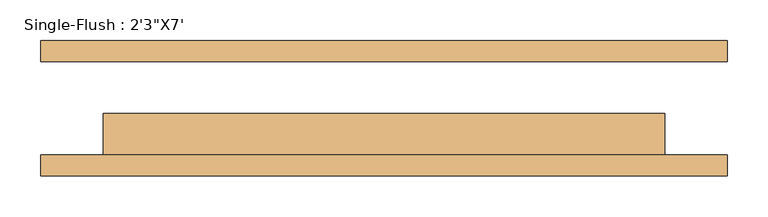
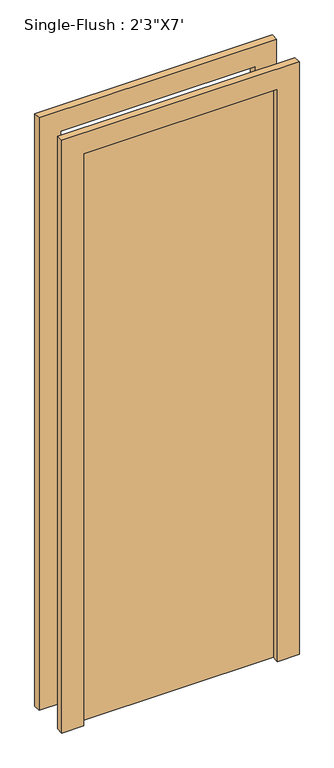
"""IFC4 building model written with IfcOpenShell, lengths in millimetres: door geometry."""

from ifc_helpers import new_model, si_unit, frame, origin, origin_with_axes, place, context, project, spatial, polyline, outline, extrude, source, transform, mapped, element, save


def door_64f31108(model_context):
    return source(origin(), model_context, "Body", "SweptSolid", [
        extrude(outline(polyline([(2209.8, -419.1), (0.0, -419.1), (0.0, -342.9), (2133.6, -342.9), (2133.6, 342.9), (0.0, 342.9), (0.0, 419.1), (2209.8, 419.1), (2209.8, -419.1)])), frame((0.0, -82.55, 0.0), z_axis=(0.0, 1.0, 0.0), x_axis=(0.0, 0.0, 1.0)), (0.0, 0.0, 1.0), 25.4),
        extrude(outline(polyline([(2209.8, 419.1), (2209.8, -419.1), (0.0, -419.1), (0.0, -342.9), (2133.6, -342.9), (2133.6, 342.9), (0.0, 342.9), (0.0, 419.1), (2209.8, 419.1)])), frame((0.0, 57.15, 0.0), z_axis=(0.0, 1.0, 0.0), x_axis=(0.0, 0.0, 1.0)), (0.0, 0.0, 1.0), 25.4),
        extrude(outline(polyline([(342.9, -6.35), (342.9, -57.15), (-342.9, -57.15), (-342.9, -6.35), (342.9, -6.35)])), origin_with_axes(), (0.0, 0.0, 1.0), 2133.6),
    ])


if __name__ == "__main__":
    model = new_model("IFC4")
    model_context = context("Model", 3, world=origin())
    ifc_project = project(units=[si_unit("LENGTHUNIT", "METRE", prefix="MILLI")], contexts=[model_context])
    site = spatial("IfcSite", under=ifc_project)
    building = spatial("IfcBuilding", under=site)
    placement = place(None, origin())
    door_shape = door_64f31108(model_context)
    element("IfcDoor", 1, ObjectType="Single-Flush : 2'3\"X7'", at=placement, inside=building, context=model_context, shape_type="MappedRepresentation", body=[
        mapped(door_shape, transform((0.0, 0.0, 0.0), x_axis=(1.0, 0.0, 0.0), y_axis=(0.0, 1.0, 0.0), z_axis=(0.0, 0.0, 1.0))),
    ])
    save(model, "model.ifc")

# Revit data of these elements
# Type "Single-Flush : 2'3\"X7'"
#   Type Mark = "10"
#   Construction Type Id = "MDOOR"
#   Assembly Code = "C1020"
#   Analytic Construction = "Metal"
#   Thickness = 0' - 2"
#   Heat Transfer Coefficient (U) = 0.651978 BTU/(h·ft²·°F)
#   Height = 7' - 0"
#   Trim Projection Ext = 0' - 1"
#   Trim Projection Int = 0' - 1"
#   Trim Width = 0' - 3"
#   Width = 2' - 3"
#   Define Thermal Properties by = 1
#   Door Material = Door - Panel
#   Frame Material = Door - Frame
#   Visual Light Transmittance = 0
#   Solar Heat Gain Coefficient = 0
#   Function = (empty or 0)
#   Wall Closure = (empty or 0)
# Element 1 (IfcDoor, "Single-Flush : 2'3\"X7'")
#   Materials on its faces: "Door - Frame", "Door - Panel"
# Materials
#   "Door - Panel": class "Wood", colour RGB 210 159 95, transparency 0, Cost = 0
#   "Door - Frame": colour RGB 118 70 51, transparency 0, Cost = 0
